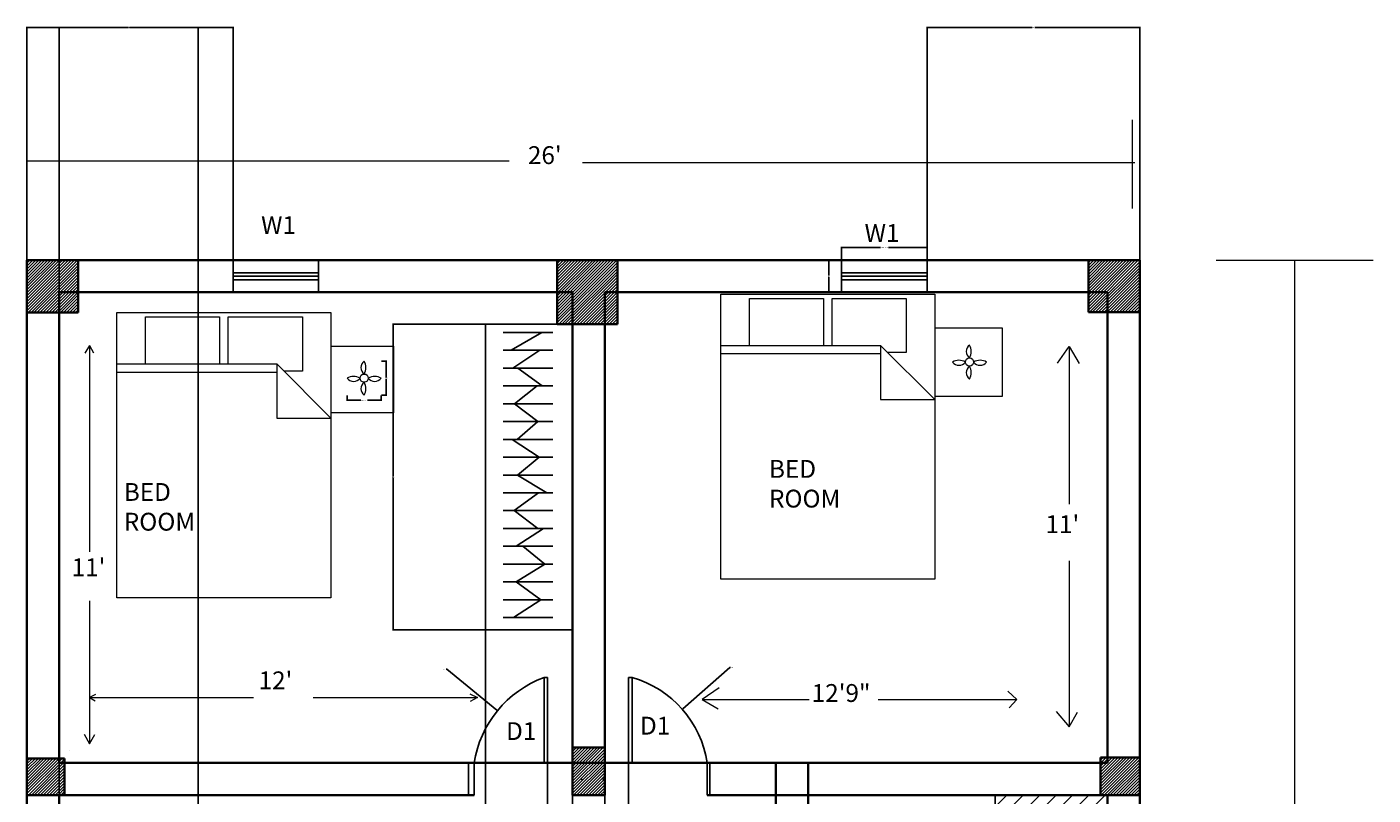
# Model space of a CAD drawing. Units: inches. Extents: x -4 to 429, y -457 to 84.
# Tile 4 of 4: x 22 to 399, y -131 to 84. Entities that reach past the tile are written whole.
import ezdxf

# ---------------------------------------------------------------- set-up
doc = ezdxf.new("R2010")
doc.units = ezdxf.units.IN
doc.header["$MEASUREMENT"] = 0
for name, color, linetype, lineweight in [('A-ANNO-DIMS', 2, 'Continuous', 18), ('A-ANNO-TEXT', 3, 'Continuous', 18), ('A-AREA-IDEN', 7, 'Continuous', 25), ('A-COLS', 7, 'Continuous', 35), ('A-COLS-PATT', 252, 'Continuous', 13), ('A-DOOR', 3, 'Continuous', 25), ('A-FLOR-CASE', 9, 'Continuous', 25), ('A-FLOR-CASE-PATT', 252, 'Continuous', 13), ('A-FURN', 8, 'Continuous', 18), ('A-GLAZ', 4, 'Continuous', 25), ('A-WALL', 7, 'Continuous', 35)]:
    doc.layers.add(name, color=color, linetype=linetype, lineweight=lineweight)
doc.styles.get("Standard").update_dxf_attribs({"font": 'arial.ttf'})
doc.dimstyles.get("Standard").update_dxf_attribs({"dimtxt": 0.18, "dimasz": 0.18, "dimexe": 0.18, "dimexo": 0.0625, "dimgap": 0.09, "dimtad": 0, "dimtih": 1, "dimtoh": 1, "dimdec": 4, "dimzin": 0, "dimdsep": 46, "dimtxsty": 'Standard', "dimcen": 0.09, "dimadec": 0, "dimazin": 0, "dimtfac": 1, "dimtdec": 4, "dimtofl": 0, "dimtmove": 0, "dimatfit": 3, "dimfxl": 1, "dimtolj": 1, "dimtzin": 0, "dimarcsym": 0})
pattern_1 = [(45, (-1330.13025, -719.5531), (-0.41542523, 0.41542523), [])]

# ---------------------------------------------------------------- blocks, each defined once
blk = doc.blocks.new('Bed - Queen')
for p, q in [((0, -80.00003), (0, 0)), ((0, 0), (59.99999, 0)), ((59.99999, 0), (59.99999, -80.00003)), ((7.99999, -1.2), (28.79998, -1.2)), ((7.99999, -14.4), (7.99999, -1.2)), ((28.79998, -1.2), (28.79998, -14.4)), ((31.19999, -1.2), (51.99999, -1.2)), ((31.19999, -14.4), (31.19999, -1.2)), ((51.99999, -1.2), (51.99999, -16.4)), ((0, -14.4), (44.8, -14.4)), ((59.99999, -29.6), (44.8, -14.4)), ((44.8, -14.4), (44.8, -29.6)), ((44.8, -16.8), (0, -16.8)), ((51.99999, -16.4), (46.79936, -16.4)), ((44.8, -29.6), (59.99999, -29.6)), ((59.99999, -80.00003), (0, -80.00003))]:
    blk.add_line(p, q)
blk = doc.blocks.new('WIN-24IN-9IN-WALL')
for p, q in [((0, 5.5), (24, 5.5)), ((0, 4.5), (24, 4.5)), ((0, 3.5), (24, 3.5))]:
    blk.add_line(p, q)
blk.add_lwpolyline([(0, 9), (24, 9), (24, 0), (0, 0)], close=True)
blk = doc.blocks.new('DOOR-LEAF-24IN')
for p, q in [((0, 0), (0, 24)), ((0, 24), (1, 24)), ((1, 24), (1, 0))]:
    blk.add_line(p, q)
blk = doc.blocks.new('BEDSIDE-FLORAL-MOTIF')
blk.add_circle((4.78, 4.78), 1.15)
for centre, radius, start, end in [((6.14, 7.74), 2.27, 126.9972, 233.0028), ((1.64, 7.74), 3.62, 330, 30), ((1.81, 1.64), 3.62, 60, 120), ((1.81, 6.14), 2.27, 216.9972, 323.0028), ((7.74, 1.64), 3.62, 60, 120), ((7.74, 6.14), 2.27, 216.9972, 323.0028), ((6.14, 1.81), 2.27, 126.9972, 233.0028), ((1.64, 1.81), 3.62, 330, 30)]:
    blk.add_arc(centre, radius, start, end)
blk = doc.blocks.new('*D12')
at = {"layer": 'A-ANNO-DIMS', "color": 0, "lineweight": -2, "transparency": 16777216}
for p, q in [((250.49, 18.72), (250.49, 22.44)), ((250.67, 22.26), (261.37, 22.26)), ((274.31, 22.26), (263.6, 22.26)), ((274.49, 18.72), (274.49, 22.44))]:
    blk.add_line(p, q, dxfattribs=at)
at = {"layer": 'A-ANNO-DIMS', "color": 0, "transparency": 16777216}
for points in [[(250.67, 22.29), (250.67, 22.23), (250.49, 22.26)], [(274.31, 22.29), (274.31, 22.23), (274.49, 22.26)]]:
    blk.add_solid(points, dxfattribs=at)
at = {"layer": 'Defpoints', "color": 0, "transparency": 16777216}
for p in [(274.49, 22.26), (250.49, 18.66), (274.49, 18.66)]:
    blk.add_point(p, dxfattribs=at)
at = {"layer": 'A-ANNO-DIMS', "color": 0, "transparency": 16777216, "insert": (262.49, 22.26), "char_height": 0.18, "attachment_point": 5}
blk.add_mtext('\\A1;WINDOW 24 TYP.', dxfattribs=at)
blk = doc.blocks.new('*D13')
at = {"layer": 'A-ANNO-DIMS', "color": 0, "lineweight": -2, "transparency": 16777216}
for p, q in [((250.42, 18.66), (246.71, 18.66)), ((246.89, 18.48), (246.89, 14.34)), ((246.89, 9.84), (246.89, 13.98)), ((250.42, 9.66), (246.71, 9.66))]:
    blk.add_line(p, q, dxfattribs=at)
at = {"layer": 'A-ANNO-DIMS', "color": 0, "transparency": 16777216}
for points in [[(246.86, 18.48), (246.92, 18.48), (246.89, 18.66)], [(246.86, 9.84), (246.92, 9.84), (246.89, 9.66)]]:
    blk.add_solid(points, dxfattribs=at)
at = {"layer": 'Defpoints', "color": 0, "transparency": 16777216}
for p in [(246.89, 18.66), (250.49, 18.66), (250.49, 9.66)]:
    blk.add_point(p, dxfattribs=at)
at = {"layer": 'A-ANNO-DIMS', "color": 0, "transparency": 16777216, "insert": (246.89, 14.16), "char_height": 0.18, "attachment_point": 5}
blk.add_mtext('\\A1;9 TYP.', dxfattribs=at)
blk = doc.blocks.new('*D22')
at = {"layer": 'A-ANNO-DIMS', "color": 0, "lineweight": -2, "transparency": 16777216}
for p, q in [((111.83, -19.24), (111.83, -20.79)), ((112.01, -20.61), (115.65, -20.61)), ((121.2, -20.61), (117.55, -20.61)), ((121.38, -19.24), (121.38, -20.79))]:
    blk.add_line(p, q, dxfattribs=at)
at = {"layer": 'A-ANNO-DIMS', "color": 0, "transparency": 16777216}
for points in [[(112.01, -20.58), (112.01, -20.64), (111.83, -20.61)], [(121.2, -20.58), (121.2, -20.64), (121.38, -20.61)]]:
    blk.add_solid(points, dxfattribs=at)
at = {"layer": 'Defpoints', "color": 0, "transparency": 16777216}
for p in [(111.83, -19.18), (121.38, -19.18), (121.38, -20.61)]:
    blk.add_point(p, dxfattribs=at)
at = {"layer": 'A-ANNO-DIMS', "color": 0, "transparency": 16777216, "insert": (116.6, -20.61), "char_height": 0.18, "attachment_point": 5}
blk.add_mtext('\\A1;MOTIF 10 TYP.', dxfattribs=at)
blk = doc.blocks.new('*D23')
at = {"layer": 'A-ANNO-DIMS', "color": 0, "lineweight": -2, "transparency": 16777216}
for p, q in [((121.44, -9.63), (122.99, -9.63)), ((122.81, -9.81), (122.81, -14.22)), ((122.81, -19), (122.81, -14.58)), ((121.44, -19.18), (122.99, -19.18))]:
    blk.add_line(p, q, dxfattribs=at)
at = {"layer": 'A-ANNO-DIMS', "color": 0, "transparency": 16777216}
for points in [[(122.78, -9.81), (122.84, -9.81), (122.81, -9.63)], [(122.78, -19), (122.84, -19), (122.81, -19.18)]]:
    blk.add_solid(points, dxfattribs=at)
at = {"layer": 'Defpoints', "color": 0, "transparency": 16777216}
for p in [(121.38, -9.63), (122.81, -9.63), (121.38, -19.18)]:
    blk.add_point(p, dxfattribs=at)
at = {"layer": 'A-ANNO-DIMS', "color": 0, "transparency": 16777216, "insert": (122.81, -14.4), "char_height": 0.18, "attachment_point": 5}
blk.add_mtext('\\A1;10 TYP.', dxfattribs=at)
blk = doc.blocks.new('*D32')
at = {"layer": 'A-ANNO-DIMS', "color": 0, "lineweight": -2, "transparency": 16777216}
for p, q in [((31.06, -294.84), (31.06, 84.09)), ((31.24, 83.91), (50.34, 83.91)), ((69.88, 83.91), (50.78, 83.91)), ((70.06, -294.84), (70.06, 84.09))]:
    blk.add_line(p, q, dxfattribs=at)
at = {"layer": 'A-ANNO-DIMS', "color": 0, "transparency": 16777216}
for points in [[(31.24, 83.94), (31.24, 83.88), (31.06, 83.91)], [(69.88, 83.94), (69.88, 83.88), (70.06, 83.91)]]:
    blk.add_solid(points, dxfattribs=at)
at = {"layer": 'Defpoints', "color": 0, "transparency": 16777216}
for p in [(70.06, 83.91), (31.06, -294.9), (70.06, -294.9)]:
    blk.add_point(p, dxfattribs=at)
at = {"layer": 'A-ANNO-DIMS', "color": 0, "transparency": 16777216, "insert": (50.56, 83.91), "char_height": 0.18, "attachment_point": 5}
blk.add_mtext('\\A1;39', dxfattribs=at)
blk = doc.blocks.new('*D34')
at = {"layer": 'A-ANNO-DIMS', "color": 0, "lineweight": -2, "transparency": 16777216}
for p, q in [((150.54, 0.74), (124.57, 0.74)), ((124.75, 0.56), (124.75, -41.95)), ((124.75, -84.83), (124.75, -42.32)), ((150.54, -85.01), (124.57, -85.01))]:
    blk.add_line(p, q, dxfattribs=at)
at = {"layer": 'A-ANNO-DIMS', "color": 0, "transparency": 16777216}
for points in [[(124.72, 0.56), (124.78, 0.56), (124.75, 0.74)], [(124.72, -84.83), (124.78, -84.83), (124.75, -85.01)]]:
    blk.add_solid(points, dxfattribs=at)
at = {"layer": 'Defpoints', "color": 0, "transparency": 16777216}
for p in [(124.75, 0.74), (150.6, 0.74), (150.6, -85.01)]:
    blk.add_point(p, dxfattribs=at)
at = {"layer": 'A-ANNO-DIMS', "color": 0, "transparency": 16777216, "insert": (124.75, -42.13), "char_height": 0.18, "attachment_point": 5}
blk.add_mtext('\\A1;85.75', dxfattribs=at)
blk = doc.blocks.new('*D35')
at = {"layer": 'A-ANNO-DIMS', "color": 0, "lineweight": -2, "transparency": 16777216}
for p, q in [((150.6, -85.07), (150.6, -457.42)), ((175.06, -85.07), (175.06, -457.42)), ((150.78, -457.24), (162.36, -457.24)), ((174.88, -457.24), (163.29, -457.24))]:
    blk.add_line(p, q, dxfattribs=at)
at = {"layer": 'A-ANNO-DIMS', "color": 0, "transparency": 16777216}
for points in [[(150.78, -457.21), (150.78, -457.27), (150.6, -457.24)], [(174.88, -457.21), (174.88, -457.27), (175.06, -457.24)]]:
    blk.add_solid(points, dxfattribs=at)
at = {"layer": 'Defpoints', "color": 0, "transparency": 16777216}
for p in [(150.6, -85.01), (175.06, -85.01), (175.06, -457.24)]:
    blk.add_point(p, dxfattribs=at)
at = {"layer": 'A-ANNO-DIMS', "color": 0, "transparency": 16777216, "insert": (162.83, -457.24), "char_height": 0.18, "attachment_point": 5}
blk.add_mtext('\\A1;24.457', dxfattribs=at)
blk = doc.blocks.new('*D38')
at = {"layer": 'A-ANNO-DIMS', "color": 0, "lineweight": -2, "transparency": 16777216}
for p, q in [((22.06, 18.72), (22.06, 84.09)), ((22.24, 83.91), (50.56, 83.91)), ((79.67, 83.91), (51.35, 83.91)), ((79.85, 18.72), (79.85, 84.09))]:
    blk.add_line(p, q, dxfattribs=at)
at = {"layer": 'A-ANNO-DIMS', "color": 0, "transparency": 16777216}
for points in [[(22.24, 83.94), (22.24, 83.88), (22.06, 83.91)], [(79.67, 83.94), (79.67, 83.88), (79.85, 83.91)]]:
    blk.add_solid(points, dxfattribs=at)
at = {"layer": 'Defpoints', "color": 0, "transparency": 16777216}
for p in [(79.85, 83.91), (22.06, 18.66), (79.85, 18.66)]:
    blk.add_point(p, dxfattribs=at)
at = {"layer": 'A-ANNO-DIMS', "color": 0, "transparency": 16777216, "insert": (50.95, 83.91), "char_height": 0.18, "attachment_point": 5}
blk.add_mtext('\\A1;57.79', dxfattribs=at)
blk = doc.blocks.new('*D39')
at = {"layer": 'A-ANNO-DIMS', "color": 0, "lineweight": -2, "transparency": 16777216}
for p, q in [((274.49, 18.72), (274.49, 84.09)), ((274.67, 83.91), (303.88, 83.91)), ((333.88, 83.91), (304.67, 83.91)), ((334.06, 18.72), (334.06, 84.09))]:
    blk.add_line(p, q, dxfattribs=at)
at = {"layer": 'A-ANNO-DIMS', "color": 0, "transparency": 16777216}
for points in [[(274.67, 83.94), (274.67, 83.88), (274.49, 83.91)], [(333.88, 83.94), (333.88, 83.88), (334.06, 83.91)]]:
    blk.add_solid(points, dxfattribs=at)
at = {"layer": 'Defpoints', "color": 0, "transparency": 16777216}
for p in [(334.06, 83.91), (274.49, 18.66), (334.06, 18.66)]:
    blk.add_point(p, dxfattribs=at)
at = {"layer": 'A-ANNO-DIMS', "color": 0, "transparency": 16777216, "insert": (304.27, 83.91), "char_height": 0.18, "attachment_point": 5}
blk.add_mtext('\\A1;59.57', dxfattribs=at)
blk = doc.blocks.new('*D51')
at = {"layer": 'A-ANNO-DIMS', "color": 0, "lineweight": -2, "transparency": 16777216}
for p, q in [((175.06, -118.1), (175.06, -457.42)), ((168.05, -122.4), (168.05, -457.42)), ((168.23, -457.24), (171.16, -457.24)), ((174.88, -457.24), (171.95, -457.24))]:
    blk.add_line(p, q, dxfattribs=at)
at = {"layer": 'A-ANNO-DIMS', "color": 0, "transparency": 16777216}
for points in [[(168.23, -457.21), (168.23, -457.27), (168.05, -457.24)], [(174.88, -457.21), (174.88, -457.27), (175.06, -457.24)]]:
    blk.add_solid(points, dxfattribs=at)
at = {"layer": 'Defpoints', "color": 0, "transparency": 16777216}
for p in [(175.06, -118.04), (168.05, -122.34), (175.06, -457.24)]:
    blk.add_point(p, dxfattribs=at)
at = {"layer": 'A-ANNO-DIMS', "color": 0, "transparency": 16777216, "insert": (171.56, -457.24), "char_height": 0.18, "attachment_point": 5}
blk.add_mtext('\\A1;7.002', dxfattribs=at)
blk = doc.blocks.new('*D52')
at = {"layer": 'A-ANNO-DIMS', "color": 0, "lineweight": -2, "transparency": 16777216}
for p, q in [((184.06, -118.1), (184.06, -457.42)), ((190.77, -122.4), (190.77, -457.42)), ((184.24, -457.24), (187.02, -457.24)), ((190.59, -457.24), (187.81, -457.24))]:
    blk.add_line(p, q, dxfattribs=at)
at = {"layer": 'A-ANNO-DIMS', "color": 0, "transparency": 16777216}
for points in [[(184.24, -457.21), (184.24, -457.27), (184.06, -457.24)], [(190.59, -457.21), (190.59, -457.27), (190.77, -457.24)]]:
    blk.add_solid(points, dxfattribs=at)
at = {"layer": 'Defpoints', "color": 0, "transparency": 16777216}
for p in [(184.06, -118.04), (190.77, -122.34), (190.77, -457.24)]:
    blk.add_point(p, dxfattribs=at)
at = {"layer": 'A-ANNO-DIMS', "color": 0, "transparency": 16777216, "insert": (187.41, -457.24), "char_height": 0.18, "attachment_point": 5}
blk.add_mtext('\\A1;6.714', dxfattribs=at)
blk = doc.blocks.new('*D55')
at = {"layer": 'A-ANNO-DIMS', "color": 0, "lineweight": -2, "transparency": 16777216}
for p, q in [((139.6, -96.07), (139.78, -96.07)), ((139.78, -96.07), (153.84, -107.56)), ((177.56, -127.01), (177.74, -127.01)), ((177.65, -127.1), (177.65, -126.92))]:
    blk.add_line(p, q, dxfattribs=at)
at = {"layer": 'A-ANNO-DIMS', "color": 0, "transparency": 16777216}
blk.add_solid([(153.86, -107.53), (153.83, -107.58), (153.98, -107.67)], dxfattribs=at)
at = {"layer": 'Defpoints', "color": 0, "transparency": 16777216}
for p in [(153.98, -107.67), (177.65, -127.01)]:
    blk.add_point(p, dxfattribs=at)
at = {"layer": 'A-ANNO-DIMS', "color": 0, "transparency": 16777216, "insert": (139.05, -96.07), "char_height": 0.18, "attachment_point": 5}
blk.add_mtext('\\A1;R30.567', dxfattribs=at)
blk = doc.blocks.new('*D56')
at = {"layer": 'A-ANNO-DIMS', "color": 0, "lineweight": -2, "transparency": 16777216}
for p, q in [((219.15, -95.57), (205.92, -107.15)), ((219.33, -95.57), (219.15, -95.57)), ((183.43, -126.77), (183.61, -126.77)), ((183.52, -126.86), (183.52, -126.68))]:
    blk.add_line(p, q, dxfattribs=at)
at = {"layer": 'A-ANNO-DIMS', "color": 0, "transparency": 16777216}
blk.add_solid([(205.9, -107.13), (205.94, -107.17), (205.79, -107.27)], dxfattribs=at)
at = {"layer": 'Defpoints', "color": 0, "transparency": 16777216}
for p in [(205.79, -107.27), (183.52, -126.77)]:
    blk.add_point(p, dxfattribs=at)
at = {"layer": 'A-ANNO-DIMS', "color": 0, "transparency": 16777216, "insert": (219.74, -95.57), "char_height": 0.18, "attachment_point": 5}
blk.add_mtext('\\A1;R29.6', dxfattribs=at)

msp = doc.modelspace()

# ---------------------------------------------------------------- hatches: boundary and pattern name
at = {"layer": 'A-COLS-PATT'}
h = msp.add_hatch(dxfattribs=at)
h.set_pattern_fill('ANSI31', color=256, scale=4.7)
h.set_pattern_definition(pattern_1)
h.paths.add_polyline_path([(36.4273, 18.6601), (22.0572, 18.6601), (22.0572, 3.9935), (31.0572, 3.9935), (31.0572, 9.6601), (36.4273, 9.6601)])
h.paths.add_polyline_path([(36.4273, 9.6601), (31.0572, 9.6601), (31.0572, 3.9935), (36.4273, 3.9935)], flags=17)
h = msp.add_hatch(dxfattribs=at)
h.set_pattern_fill('ANSI31', color=256, scale=4.7)
h.set_pattern_definition(pattern_1)
h.paths.add_polyline_path([(187.6253, 18.6601), (170.7464, 18.6601), (170.7464, 9.6601), (175.0572, 9.6601), (175.0572, 0.7407), (184.0572, 0.7407), (184.0572, 9.6601), (187.6253, 9.6601)])
h.paths.add_polyline_path([(175.0572, 9.6601), (170.7464, 9.6601), (170.7464, 0.7407), (175.0572, 0.7407)], flags=17)
h.paths.add_polyline_path([(187.6253, 9.6601), (184.0572, 9.6601), (184.0572, 0.7407), (187.6253, 0.7407)])
h = msp.add_hatch(dxfattribs=at)
h.set_pattern_fill('ANSI31', color=256, scale=4.7)
h.set_pattern_definition(pattern_1)
h.paths.add_polyline_path([(334.0572, 18.6601), (319.6894, 18.6601), (319.6894, 9.6601), (325.0572, 9.6601), (325.0572, 4.1221), (334.0572, 4.1221)])
h.paths.add_polyline_path([(325.0572, 9.6601), (319.6894, 9.6601), (319.6894, 4.1221), (325.0572, 4.1221)], flags=17)
h = msp.add_hatch(dxfattribs=at)
h.set_pattern_fill('ANSI31', color=256, scale=4.7)
h.set_pattern_definition(pattern_1)
h.paths.add_polyline_path([(184.0572, -122.3399), (175.0572, -122.3399), (175.0572, -131.3399), (184.0572, -131.3399)])
h.paths.add_polyline_path([(184.0572, -118.0379), (175.0572, -118.0379), (175.0572, -122.3399), (184.0572, -122.3399)])
h = msp.add_hatch(dxfattribs=at)
h.set_pattern_fill('ANSI31', color=256, scale=4.7)
h.set_pattern_definition(pattern_1)
h.paths.add_polyline_path([(325.0572, -120.7565), (323.0368, -120.7565), (323.0368, -122.3399), (325.0572, -122.3399)], flags=17)
h.paths.add_polyline_path([(334.0572, -120.7565), (325.0572, -120.7565), (325.0572, -122.3399), (323.0368, -122.3399), (323.0368, -131.3399), (325.0572, -131.3399), (334.0572, -131.3399)])
h = msp.add_hatch(dxfattribs=at)
h.set_pattern_fill('ANSI31', color=256, scale=4.7)
h.set_pattern_definition(pattern_1)
h.paths.add_polyline_path([(32.5781, -122.3399), (31.0572, -122.3399), (31.0572, -121.0524), (22.0572, -121.0524), (22.0572, -131.3399), (32.5781, -131.3399)])
h.paths.add_polyline_path([(32.5781, -121.0524), (31.0572, -121.0524), (31.0572, -122.3399), (32.5781, -122.3399)], flags=17)
at = {"layer": 'A-FLOR-CASE-PATT'}
h = msp.add_hatch(dxfattribs=at)
h.set_pattern_fill('ANSI31', color=256, scale=26)
h.set_pattern_definition([(45, (-1330.1303, -719.553), (-2.298097, 2.298097), [])])
h.paths.add_polyline_path([(325.0572, -131.3399), (293.5167, -131.3399), (293.5167, -216.4188), (241.0572, -216.4188), (241.0572, -251.3399), (325.0572, -251.3399)])

# ---------------------------------------------------------------- linework, layer by layer
at = {"layer": 'A-ANNO-DIMS'}
for p, q in [((22.0572, 35.7887), (22.0572, 57.333)), ((331.9552, 58.0633), (331.9552, 33.209)), ((22.0572, 46.5609), (157.2374, 46.5609)), ((177.8264, 46.0713), (332.7348, 46.0713)), ((355.4886, 18.6601), (399.4889, 18.6601)), ((377.4887, 18.6601), (377.4887, -176.2694)), ((39.5621, -5.2696), (38.3291, -7.4054)), ((39.5621, -5.2696), (39.5621, -63.1241)), ((39.5621, -5.2696), (40.745, -7.3183)), ((311.0442, -10.2375), (314.2694, -5.5034)), ((314.2694, -5.5034), (314.2694, -49.7816)), ((314.2694, -5.5034), (317.0473, -10.3149)), ((314.2694, -65.6492), (314.2694, -112.2377)), ((39.5621, -76.8806), (39.5621, -116.9337)), ((216.1683, -101.2324), (211.3433, -104.5371)), ((41.2881, -103.1544), (39.5621, -103.9535)), ((39.5621, -103.9535), (85.6026, -103.9535)), ((39.5621, -103.9535), (41.1746, -104.8844)), ((102.311, -103.9535), (148.3517, -103.9535)), ((146.2541, -102.9617), (148.3517, -103.9535)), ((148.3517, -103.9535), (146.3572, -105.1051)), ((211.3433, -104.5371), (241.4107, -104.5371)), ((211.3433, -104.5371), (215.8545, -107.1416)), ((260.6847, -104.5371), (299.6181, -104.5371)), ((297.0449, -102.1934), (299.6181, -104.5371)), ((299.6181, -104.5371), (297.4651, -106.9009)), ((310.651, -107.9189), (314.2694, -112.2377)), ((314.2694, -112.2377), (316.6589, -108.099)), ((38.1492, -114.2876), (39.5621, -116.9337)), ((39.5621, -116.9337), (41.0523, -114.3526))]:
    msp.add_line(p, q, dxfattribs=at)
at = {"layer": 'A-COLS'}
for p, q in [((36.4273, 18.6601), (36.4273, 3.9935)), ((170.7464, 18.6601), (170.7464, 0.7407)), ((187.6253, 18.6601), (170.7464, 18.6601)), ((187.6253, 0.7407), (187.6253, 18.6601)), ((319.6894, 18.6601), (319.6894, 4.1221)), ((36.4273, 3.9935), (22.0572, 3.9935)), ((319.6894, 4.1221), (334.0572, 4.1221)), ((170.7464, 0.7407), (187.6253, 0.7407)), ((33.957, -118.8722), (33.957, -118.8722)), ((175.0572, -118.0379), (184.0572, -118.0379)), ((334.0572, -120.7565), (323.0368, -120.7565)), ((323.0368, -120.7565), (323.0368, -131.3399)), ((22.0572, -121.0524), (32.5781, -121.0524)), ((32.5781, -121.0524), (32.5781, -131.3399)), ((38.7181, -131.3399), (22.0572, -131.3399)), ((175.0572, -131.3399), (184.0572, -131.3399)), ((325.0572, -131.3399), (334.0572, -131.3399))]:
    msp.add_line(p, q, dxfattribs=at)
at = {"layer": 'A-DOOR'}
for p, q in [((145.8213, -122.3399), (145.8213, -131.3399)), ((147.4463, -122.3399), (147.4463, -131.3399)), ((212.7849, -122.3399), (212.7849, -131.3399)), ((213.5669, -122.3399), (213.5669, -131.3399))]:
    msp.add_line(p, q, dxfattribs=at)
for centre, radius, start, end in [((177.654, -127.01), 30.5666, 110.28898, 171.21163), ((183.5179, -126.7657), 29.5997, 8.599294, 73.809713)]:
    msp.add_arc(centre, radius, start, end, dxfattribs=at)
at = {"layer": 'A-FLOR-CASE'}
for p, q in [((170.7464, 0.7407), (150.6, 0.7407)), ((150.6, 0.7407), (150.6, -85.0072)), ((155.6185, -1.5748), (169.4931, -1.5748)), ((166.3989, -1.5748), (157.8201, -6.5748)), ((155.6185, -6.5748), (169.4931, -6.5748)), ((165.8193, -6.5748), (158.2838, -11.5748)), ((155.6185, -11.5748), (169.4931, -11.5748)), ((159.675, -11.5748), (166.5148, -16.5748)), ((155.6185, -16.5748), (169.4931, -16.5748)), ((158.7927, -21.5748), (165.0945, -16.5748)), ((155.6185, -21.5748), (169.4931, -21.5748)), ((158.7927, -21.5748), (165.3279, -26.5748)), ((155.6185, -26.5748), (169.4931, -26.5748)), ((165.3279, -26.5748), (159.4929, -31.5748)), ((155.6185, -31.5748), (169.4931, -31.5748)), ((158.0925, -31.5748), (165.678, -36.5748)), ((155.6185, -36.5748), (169.4931, -36.5748)), ((165.678, -36.5748), (159.5816, -41.5748)), ((155.6185, -41.5748), (169.4931, -41.5748)), ((159.5816, -41.5748), (167.8229, -46.5748)), ((155.6185, -46.5748), (169.4931, -46.5748)), ((165.469, -46.5748), (158.6405, -51.5748)), ((155.6185, -51.5748), (169.4931, -51.5748)), ((158.6405, -51.5748), (165.3513, -56.5748)), ((155.6185, -56.5748), (169.4931, -56.5748)), ((166.8816, -56.5748), (159.2289, -61.5748)), ((155.6185, -61.5748), (169.4931, -61.5748)), ((161.1127, -61.5748), (167.2348, -66.5748)), ((155.6185, -66.5748), (169.4931, -66.5748)), ((167.2348, -66.5748), (159.2289, -71.5748)), ((155.6185, -71.5748), (169.4931, -71.5748)), ((159.2289, -71.5748), (166.1752, -76.5748)), ((155.6185, -76.5748), (169.4931, -76.5748)), ((166.1752, -76.5748), (158.5225, -81.5748)), ((155.6185, -81.5748), (169.4931, -81.5748)), ((150.6, -85.0072), (175.0572, -85.0072)), ((293.5167, -131.3399), (293.5167, -216.4188))]:
    msp.add_line(p, q, dxfattribs=at)
at = {"layer": 'A-FURN'}
for p, q in [((276.6093, -0.2587), (295.4647, -0.2587)), ((295.4647, -0.2587), (295.4647, -19.5351)), ((107.2908, -5.4366), (124.8391, -5.4366)), ((124.8391, -5.4366), (124.8391, -24.0987)), ((295.4647, -19.5351), (276.6093, -19.5351)), ((124.8391, -24.0987), (107.2908, -24.0987))]:
    msp.add_line(p, q, dxfattribs=at)
at = {"layer": 'A-WALL'}
for p, q in [((31.0572, 9.6601), (175.0572, 9.6601)), ((31.0572, -122.3399), (31.0572, 9.6601)), ((175.0572, -131.3399), (175.0572, 9.6601)), ((184.0572, -131.3399), (184.0572, 9.6601)), ((184.0572, 9.6601), (325.0572, 9.6601)), ((325.0572, 9.6601), (325.0572, -122.3399)), ((31.0572, -122.3399), (325.0572, -122.3399)), ((232.0572, -251.3399), (232.0572, -122.3399)), ((241.0572, -251.3399), (241.0572, -122.3399)), ((31.0572, -131.3399), (147.4463, -131.3399)), ((31.0572, -251.3399), (31.0572, -131.3399)), ((212.7849, -131.3399), (325.0572, -131.3399)), ((325.0572, -131.3399), (325.0572, -251.3399))]:
    msp.add_line(p, q, dxfattribs=at)
msp.add_lwpolyline([(22.0572, 18.6601), (334.0572, 18.6601), (334.0572, -431.3399), (22.0572, -431.3399)], close=True, dxfattribs=at)

# ---------------------------------------------------------------- block references
at = {"layer": 'A-DOOR'}
for p in [(167.0547, -122.34), (190.771, -122.34)]:
    msp.add_blockref('DOOR-LEAF-24IN', p, dxfattribs=at)
at = {"layer": 'A-FURN'}
for name, p in [('Bed - Queen', (216.6093, 9.1699)), ('Bed - Queen', (47.2908, 3.9935)), ('BEDSIDE-FLORAL-MOTIF', (281.568, -14.673)), ('BEDSIDE-FLORAL-MOTIF', (111.8287, -19.1785))]:
    msp.add_blockref(name, p, dxfattribs=at)
at = {"layer": 'A-GLAZ'}
for p in [(79.849, 9.66), (250.4857, 9.66)]:
    msp.add_blockref('WIN-24IN-9IN-WALL', p, dxfattribs=at)

# ---------------------------------------------------------------- texts
at = {"layer": 'A-ANNO-DIMS', "char_height": 5, "attachment_point": 1}
for s, width, insert in [("26'", 16.389113, (162.5195, 50.631)), ("11'", 14.089326, (307.641, -52.8577)), ("11'", 8.118458, (34.5927, -64.9447)), ("12'", 9.623569, (87.0115, -96.662)), ('12\'9"', 16.147427, (242.0853, -100.2119))]:
    msp.add_mtext_dynamic_manual_height_columns(s, width=width, gutter_width=25, heights=[0], dxfattribs=dict(at, insert=insert))
at = {"layer": 'A-ANNO-TEXT', "char_height": 5, "attachment_point": 1}
for s, width, insert in [('W1 ', 20.307174, (87.7118, 31.0167)), ('W1', 19.96872, (256.9263, 28.7823)), ('D1', 10.479482, (193.9498, -109.3713)), ('D1', 6.918494, (156.4068, -110.8956))]:
    msp.add_mtext_dynamic_manual_height_columns(s, width=width, gutter_width=25, heights=[0], dxfattribs=dict(at, insert=insert))
at = {"layer": 'A-AREA-IDEN', "char_height": 5, "attachment_point": 1}
for width, insert in [(22.155598, (230.1206, -37.3632)), (22.319361, (49.221, -43.8335))]:
    msp.add_mtext_dynamic_manual_height_columns('BED ROOM', width=width, gutter_width=25, heights=[0], dxfattribs=dict(at, insert=insert))

# ---------------------------------------------------------------- dimensions: what is measured, and where the dimension line sits
at = {"layer": 'A-ANNO-DIMS'}
for base, p1, p2, override, picture, middle in [((79.8489, 83.9133), (22.0572, 18.6601), (79.8489, 18.6601), {"dimdec": 2, "dimlfac": 1, "dimrnd": 0, "dimzin": 0, "dimdsep": 46, "dimlunit": 2}, '*D38', (50.9531, 83.9133)), ((70.0572, 83.9133), (31.0572, -294.9035), (70.0572, -294.9035), {"dimdec": 0, "dimlfac": 1, "dimrnd": 0, "dimzin": 0, "dimdsep": 46, "dimlunit": 2}, '*D32', (50.5572, 83.9133)), ((334.0572, 83.9133), (274.4856, 18.6601), (334.0572, 18.6601), {"dimdec": 2, "dimlfac": 1, "dimrnd": 0, "dimzin": 0, "dimdsep": 46, "dimlunit": 2}, '*D39', (304.2714, 83.9133)), ((175.0572, -457.2361), (150.6, -85.0072), (175.0572, -85.0072), {"dimdec": 3, "dimlfac": 1, "dimrnd": 0, "dimzin": 0, "dimdsep": 46, "dimlunit": 2}, '*D35', (162.8286, -457.2361)), ((175.0572, -457.2361), (168.0549, -122.3399), (175.0572, -118.0379), {"dimdec": 3, "dimlfac": 1, "dimrnd": 0, "dimzin": 0, "dimdsep": 46, "dimlunit": 2}, '*D51', (171.5561, -457.2361)), ((190.7712, -457.2361), (184.0572, -118.0379), (190.7712, -122.3399), {"dimdec": 3, "dimlfac": 1, "dimrnd": 0, "dimzin": 0, "dimdsep": 46, "dimlunit": 2}, '*D52', (187.4142, -457.2361))]:
    dim = msp.add_linear_dim(base=base, p1=p1, p2=p2, dimstyle='Standard', override=override, dxfattribs=at)
    dim.commit()
    dim.dimension.update_dxf_attribs({"geometry": picture, "text_midpoint": middle})
for base, p1, p2, text, picture, middle in [((274.4856, 22.2601), (250.4856, 18.6601), (274.4856, 18.6601), 'WINDOW <> TYP.', '*D12', (262.4856, 22.2601)), ((121.3803, -20.611), (111.8286, -19.1782), (121.3803, -19.1782), 'MOTIF <> TYP.', '*D22', (116.6045, -20.611))]:
    dim = msp.add_linear_dim(base=base, p1=p1, p2=p2, text=text, dimstyle='Standard', override={"dimdec": 0, "dimlfac": 1, "dimrnd": 0, "dimzin": 0, "dimdsep": 46, "dimlunit": 2}, dxfattribs=at)
    dim.commit()
    dim.dimension.update_dxf_attribs({"geometry": picture, "text_midpoint": middle})
for base, p1, p2, picture, middle in [((246.8856, 18.6601), (250.4856, 9.6601), (250.4856, 18.6601), '*D13', (246.8856, 14.1601)), ((122.8131, -9.6265), (121.3803, -19.1782), (121.3803, -9.6265), '*D23', (122.8131, -14.4024))]:
    dim = msp.add_linear_dim(base=base, p1=p1, p2=p2, angle=90, text='<> TYP.', dimstyle='Standard', override={"dimdec": 0, "dimlfac": 1, "dimrnd": 0, "dimzin": 0, "dimdsep": 46, "dimlunit": 2}, dxfattribs=at)
    dim.commit()
    dim.dimension.update_dxf_attribs({"geometry": picture, "text_midpoint": middle})
dim = msp.add_linear_dim(base=(124.75, 0.7407), p1=(150.6, -85.0072), p2=(150.6, 0.7407), angle=90, dimstyle='Standard', override={"dimdec": 2, "dimlfac": 1, "dimrnd": 0, "dimzin": 0, "dimdsep": 46, "dimlunit": 2}, dxfattribs=at)
dim.commit()
dim.dimension.update_dxf_attribs({"geometry": '*D34', "text_midpoint": (124.75, -42.1332)})
for center, mpoint, override, picture, middle in [((177.654, -127.01), (153.9834, -107.6704), {"dimdec": 3, "dimlfac": 1, "dimrnd": 0, "dimzin": 0, "dimdsep": 46, "dimlunit": 2}, '*D55', (139.0513, -96.0666)), ((183.5179, -126.7657), (205.7878, -107.2671), {"dimdec": 1, "dimlfac": 1, "dimrnd": 0, "dimzin": 0, "dimdsep": 46, "dimlunit": 2}, '*D56', (219.7396, -95.568))]:
    dim = msp.add_radius_dim(center=center, mpoint=mpoint, dimstyle='Standard', override=override, dxfattribs=at)
    dim.commit()
    dim.dimension.update_dxf_attribs({"geometry": picture, "text_midpoint": middle, "dimtype": 164})

doc.saveas('drawing.dxf')
